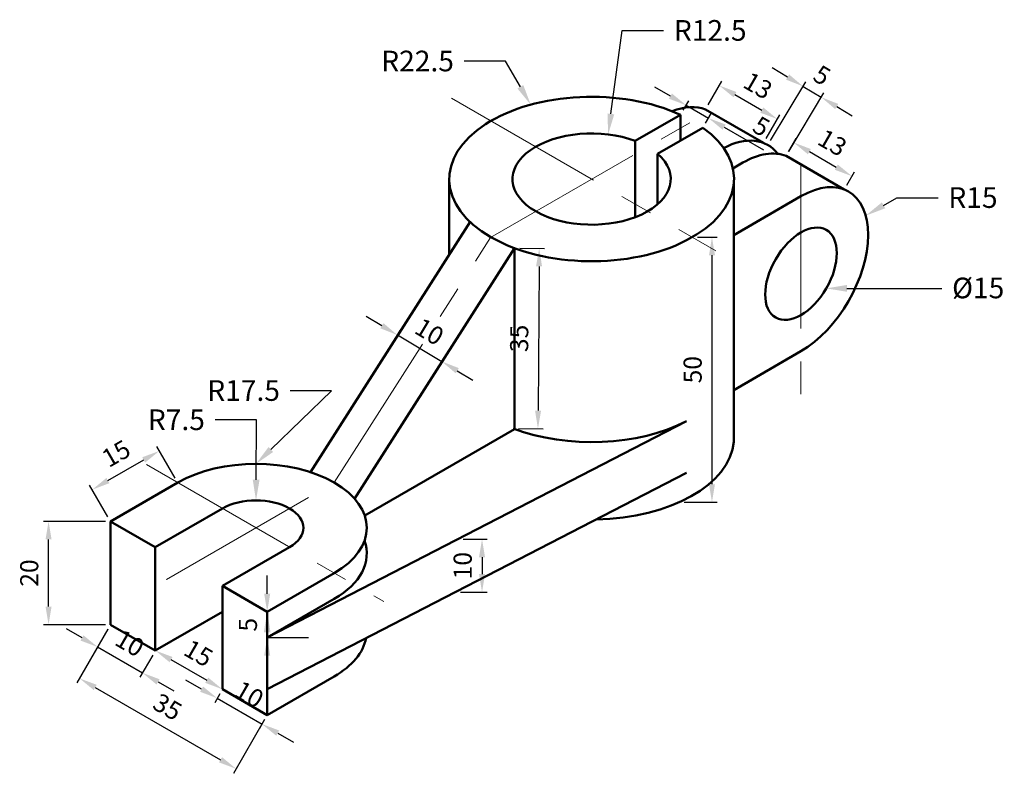
# Model space of a CAD drawing. Units: millimetres. Extents: x 2510 to 2700, y 1178 to 1324.
import ezdxf
from ezdxf import colors
from ezdxf.entities.mleader import LeaderData, LeaderLine
from ezdxf.math import Vec2, Vec3

# ---------------------------------------------------------------- set-up
doc = ezdxf.new("R2010")
doc.units = ezdxf.units.MM
doc.linetypes.add('CENTER', pattern=[50.8, 31.75, -6.35, 6.35, -6.35])
for name, color, linetype, lineweight in [('M-CNTR', 1, 'CENTER', 18), ('M-DIMS', 3, 'Continuous', 25), ('M-OUTL', 7, 'Continuous', 50)]:
    doc.layers.add(name, color=color, linetype=linetype, lineweight=lineweight)
doc.styles.get("Standard").update_dxf_attribs({"font": 'arial.ttf'})
doc.dimstyles.new('AM_ISO$0', dxfattribs={"dimtxt": 3.5, "dimasz": 3.5, "dimexe": 1, "dimexo": 1, "dimgap": 1.5, "dimtad": 1, "dimdsep": 46, "dimtxsty": 'Standard', "dimcen": 0, "dimclrd": 256, "dimclre": 256, "dimclrt": 2, "dimadec": 0, "dimazin": 2, "dimtp": 0.1, "dimtm": 0.1, "dimtfac": 0.71, "dimtdec": 3, "dimtmove": 0, "dimatfit": 3, "dimfxl": 1, "dimlwd": -1, "dimlwe": -1, "dimarcsym": 1})

# ---------------------------------------------------------------- blocks, each defined once
blk = doc.blocks.new('*D3')
at = {"layer": 'Defpoints', "color": 0, "transparency": 16777216}
for p in [(2640.08, 1281.6), (2637.52, 1230.3), (2643.88, 1230.3)]:
    blk.add_point(p, dxfattribs=at)
at = {"layer": 'M-DIMS', "color": 0, "linetype": 'ByBlock', "transparency": 16777216}
for p, q in [((2641.08, 1281.6), (2644.88, 1281.6)), ((2643.88, 1278.1), (2643.88, 1233.8)), ((2638.52, 1230.3), (2644.88, 1230.3))]:
    blk.add_line(p, q, dxfattribs=at)
at = {"layer": 'M-DIMS', "color": 0, "transparency": 16777216}
for points in [[(2643.3, 1278.1), (2644.46, 1278.1), (2643.88, 1281.6)], [(2643.3, 1233.8), (2644.46, 1233.8), (2643.88, 1230.3)]]:
    blk.add_solid(points, dxfattribs=at)
at = {"layer": 'M-DIMS', "color": 0, "transparency": 16777216, "insert": (2640.59, 1255.95), "char_height": 3.5, "attachment_point": 5, "rotation": 90}
blk.add_mtext('50', dxfattribs=at)
blk = doc.blocks.new('*D4')
at = {"layer": 'Defpoints', "color": 0, "transparency": 16777216}
for p in [(2605.68, 1279.48), (2605.44, 1244.57), (2610.2, 1244.53)]:
    blk.add_point(p, dxfattribs=at)
at = {"layer": 'M-DIMS', "color": 0, "linetype": 'ByBlock', "transparency": 16777216}
for p, q in [((2606.68, 1279.47), (2611.44, 1279.44)), ((2610.41, 1275.94), (2610.22, 1248.03)), ((2606.44, 1244.56), (2611.2, 1244.53))]:
    blk.add_line(p, q, dxfattribs=at)
at = {"layer": 'M-DIMS', "color": 0, "transparency": 16777216}
for points in [[(2609.83, 1275.95), (2611, 1275.94), (2610.44, 1279.44)], [(2609.64, 1248.04), (2610.81, 1248.03), (2610.2, 1244.53)]]:
    blk.add_solid(points, dxfattribs=at)
at = {"layer": 'M-DIMS', "color": 0, "transparency": 16777216, "insert": (2607.03, 1262.01), "char_height": 3.5, "attachment_point": 5, "rotation": 89.6095}
blk.add_mtext('35', dxfattribs=at)
blk = doc.blocks.new('*D5')
at = {"layer": 'Defpoints', "color": 0, "transparency": 16777216}
for p in [(2515.5, 1226.6), (2527.5, 1226.6), (2527.5, 1206.6)]:
    blk.add_point(p, dxfattribs=at)
at = {"layer": 'M-DIMS', "color": 0, "linetype": 'ByBlock', "transparency": 16777216}
for p, q in [((2526.5, 1226.6), (2514.5, 1226.6)), ((2515.5, 1210.1), (2515.5, 1223.1)), ((2526.5, 1206.6), (2514.5, 1206.6))]:
    blk.add_line(p, q, dxfattribs=at)
at = {"layer": 'M-DIMS', "color": 0, "transparency": 16777216}
for points in [[(2514.91, 1223.1), (2516.08, 1223.1), (2515.5, 1226.6)], [(2514.91, 1210.1), (2516.08, 1210.1), (2515.5, 1206.6)]]:
    blk.add_solid(points, dxfattribs=at)
at = {"layer": 'M-DIMS', "color": 0, "transparency": 16777216, "insert": (2512.21, 1216.6), "char_height": 3.5, "attachment_point": 5, "rotation": 90}
blk.add_mtext('20', dxfattribs=at)
blk = doc.blocks.new('*D6')
at = {"layer": 'Defpoints', "color": 0, "transparency": 16777216}
for p in [(2527.5, 1206.6), (2536.16, 1201.6), (2533.66, 1197.29)]:
    blk.add_point(p, dxfattribs=at)
at = {"layer": 'M-DIMS', "color": 0, "linetype": 'ByBlock', "transparency": 16777216}
for p, q in [((2521.97, 1204.04), (2518.94, 1205.79)), ((2527, 1205.74), (2524.5, 1201.42)), ((2525, 1202.29), (2533.66, 1197.29)), ((2535.66, 1200.74), (2533.16, 1196.42)), ((2536.69, 1195.54), (2539.73, 1193.79))]:
    blk.add_line(p, q, dxfattribs=at)
at = {"layer": 'M-DIMS', "color": 0, "transparency": 16777216}
for points in [[(2522.26, 1204.54), (2521.68, 1203.53), (2525, 1202.29)], [(2536.99, 1196.04), (2536.4, 1195.03), (2533.66, 1197.29)]]:
    blk.add_solid(points, dxfattribs=at)
at = {"layer": 'M-DIMS', "color": 0, "transparency": 16777216, "insert": (2530.98, 1202.63), "char_height": 3.5, "attachment_point": 5, "rotation": 330}
blk.add_mtext('10', dxfattribs=at)
blk = doc.blocks.new('*D7')
at = {"layer": 'Defpoints', "color": 0, "transparency": 16777216}
for p in [(2536.16, 1201.6), (2549.15, 1194.1), (2549.15, 1194.1)]:
    blk.add_point(p, dxfattribs=at)
at = {"layer": 'M-DIMS', "color": 0, "linetype": 'ByBlock', "transparency": 16777216}
blk.add_line((2539.19, 1199.85), (2546.12, 1195.85), dxfattribs=at)
at = {"layer": 'M-DIMS', "color": 0, "transparency": 16777216}
for points in [[(2539.48, 1200.36), (2538.9, 1199.35), (2536.16, 1201.6)], [(2546.41, 1196.36), (2545.82, 1195.35), (2549.15, 1194.1)]]:
    blk.add_solid(points, dxfattribs=at)
at = {"layer": 'M-DIMS', "color": 0, "transparency": 16777216, "insert": (2544.29, 1200.7), "char_height": 3.5, "attachment_point": 5, "rotation": 330}
blk.add_mtext('15', dxfattribs=at)
blk = doc.blocks.new('*D8')
at = {"layer": 'Defpoints', "color": 0, "transparency": 16777216}
for p in [(2549.15, 1194.1), (2557.81, 1189.1), (2556.81, 1187.37)]:
    blk.add_point(p, dxfattribs=at)
at = {"layer": 'M-DIMS', "color": 0, "linetype": 'ByBlock', "transparency": 16777216}
for p, q in [((2545.12, 1194.12), (2542.08, 1195.87)), ((2548.65, 1193.24), (2547.65, 1191.51)), ((2548.15, 1192.37), (2556.81, 1187.37)), ((2557.31, 1188.24), (2556.31, 1186.51)), ((2559.84, 1185.62), (2562.87, 1183.87))]:
    blk.add_line(p, q, dxfattribs=at)
at = {"layer": 'M-DIMS', "color": 0, "transparency": 16777216}
for points in [[(2545.41, 1194.63), (2544.82, 1193.62), (2548.15, 1192.37)], [(2560.13, 1186.13), (2559.55, 1185.12), (2556.81, 1187.37)]]:
    blk.add_solid(points, dxfattribs=at)
at = {"layer": 'M-DIMS', "color": 0, "transparency": 16777216, "insert": (2554.12, 1192.72), "char_height": 3.5, "attachment_point": 5, "rotation": 330}
blk.add_mtext('10', dxfattribs=at)
blk = doc.blocks.new('*D9')
at = {"layer": 'Defpoints', "color": 0, "transparency": 16777216}
for p in [(2527.5, 1206.6), (2557.81, 1189.1), (2551.81, 1178.71)]:
    blk.add_point(p, dxfattribs=at)
at = {"layer": 'M-DIMS', "color": 0, "linetype": 'ByBlock', "transparency": 16777216}
for p, q in [((2527, 1205.74), (2521, 1195.34)), ((2524.53, 1194.46), (2548.78, 1180.46)), ((2557.31, 1188.24), (2551.31, 1177.84))]:
    blk.add_line(p, q, dxfattribs=at)
at = {"layer": 'M-DIMS', "color": 0, "transparency": 16777216}
for points in [[(2524.82, 1194.97), (2524.24, 1193.96), (2521.5, 1196.21)], [(2549.07, 1180.97), (2548.48, 1179.96), (2551.81, 1178.71)]]:
    blk.add_solid(points, dxfattribs=at)
at = {"layer": 'M-DIMS', "color": 0, "transparency": 16777216, "insert": (2538.3, 1190.31), "char_height": 3.5, "attachment_point": 5, "rotation": 330}
blk.add_mtext('35', dxfattribs=at)
blk = doc.blocks.new('*D10')
at = {"layer": 'Defpoints', "color": 0, "transparency": 16777216}
for p in [(2536.94, 1240.24), (2540.49, 1234.1), (2527.5, 1226.6)]:
    blk.add_point(p, dxfattribs=at)
at = {"layer": 'M-DIMS', "color": 0, "linetype": 'ByBlock', "transparency": 16777216}
for p, q in [((2539.99, 1234.97), (2536.44, 1241.11)), ((2526.98, 1234.49), (2533.91, 1238.49)), ((2527, 1227.47), (2523.45, 1233.61))]:
    blk.add_line(p, q, dxfattribs=at)
at = {"layer": 'M-DIMS', "color": 0, "transparency": 16777216}
for points in [[(2533.62, 1239), (2534.2, 1237.99), (2536.94, 1240.24)], [(2526.69, 1235), (2527.27, 1233.99), (2523.95, 1232.74)]]:
    blk.add_solid(points, dxfattribs=at)
at = {"layer": 'M-DIMS', "color": 0, "transparency": 16777216, "insert": (2528.8, 1239.34), "char_height": 3.5, "attachment_point": 5, "rotation": 30}
blk.add_mtext('15', dxfattribs=at)
blk = doc.blocks.new('*D11')
at = {"layer": 'Defpoints', "color": 0, "transparency": 16777216}
for p in [(2581.62, 1260.35), (2591.59, 1257.55), (2590.2, 1255.23)]:
    blk.add_point(p, dxfattribs=at)
at = {"layer": 'M-DIMS', "color": 0, "linetype": 'ByBlock', "transparency": 16777216}
for p, q in [((2580, 1264.46), (2576.99, 1266.26)), ((2582.13, 1261.21), (2583.52, 1263.53)), ((2583, 1262.67), (2591.59, 1257.55)), ((2590.72, 1256.09), (2592.1, 1258.41)), ((2594.59, 1255.76), (2597.6, 1253.96))]:
    blk.add_line(p, q, dxfattribs=at)
at = {"layer": 'M-DIMS', "color": 0, "transparency": 16777216}
for points in [[(2580.3, 1264.96), (2579.7, 1263.96), (2583, 1262.67)], [(2594.89, 1256.26), (2594.29, 1255.26), (2591.59, 1257.55)]]:
    blk.add_solid(points, dxfattribs=at)
at = {"layer": 'M-DIMS', "color": 0, "transparency": 16777216, "insert": (2588.98, 1262.93), "char_height": 3.5, "attachment_point": 5, "rotation": 329.1839}
blk.add_mtext('10', dxfattribs=at)
blk = doc.blocks.new('*D12')
at = {"layer": 'Defpoints', "color": 0, "transparency": 16777216}
for p in [(2637.79, 1305.28), (2643.2, 1304.65), (2642.12, 1302.78)]:
    blk.add_point(p, dxfattribs=at)
at = {"layer": 'M-DIMS', "color": 0, "linetype": 'ByBlock', "transparency": 16777216}
for p, q in [((2635.84, 1308.9), (2632.81, 1310.65)), ((2638.29, 1306.15), (2639.37, 1308.01)), ((2638.87, 1307.15), (2643.2, 1304.65)), ((2642.62, 1303.65), (2643.7, 1305.51)), ((2646.23, 1302.9), (2653.87, 1298.49))]:
    blk.add_line(p, q, dxfattribs=at)
at = {"layer": 'M-DIMS', "color": 0, "transparency": 16777216}
for points in [[(2636.13, 1309.4), (2635.55, 1308.39), (2638.87, 1307.15)], [(2646.52, 1303.4), (2645.94, 1302.39), (2643.2, 1304.65)]]:
    blk.add_solid(points, dxfattribs=at)
at = {"layer": 'M-DIMS', "color": 0, "transparency": 16777216, "insert": (2653.21, 1302.66), "char_height": 3.5, "attachment_point": 5, "rotation": 330}
blk.add_mtext('5', dxfattribs=at)
blk = doc.blocks.new('*D13')
at = {"layer": 'Defpoints', "color": 0, "transparency": 16777216}
for p in [(2642.62, 1306.33), (2656.54, 1304.45), (2653.88, 1299.83)]:
    blk.add_point(p, dxfattribs=at)
at = {"layer": 'M-DIMS', "color": 0, "linetype": 'ByBlock', "transparency": 16777216}
for p, q in [((2643.12, 1307.19), (2645.79, 1311.81)), ((2648.32, 1309.2), (2653.51, 1306.2)), ((2654.38, 1300.69), (2657.04, 1305.31))]:
    blk.add_line(p, q, dxfattribs=at)
at = {"layer": 'M-DIMS', "color": 0, "transparency": 16777216}
for points in [[(2648.61, 1309.7), (2648.03, 1308.69), (2645.29, 1310.95)], [(2653.81, 1306.7), (2653.22, 1305.69), (2656.54, 1304.45)]]:
    blk.add_solid(points, dxfattribs=at)
at = {"layer": 'M-DIMS', "color": 0, "transparency": 16777216, "insert": (2652.56, 1310.54), "char_height": 3.5, "attachment_point": 5, "rotation": 330}
blk.add_mtext('13', dxfattribs=at)
blk = doc.blocks.new('*D14')
at = {"layer": 'Defpoints', "color": 0, "transparency": 16777216}
for p in [(2658.21, 1297.33), (2670.96, 1293.41), (2669.47, 1290.83)]:
    blk.add_point(p, dxfattribs=at)
at = {"layer": 'M-DIMS', "color": 0, "linetype": 'ByBlock', "transparency": 16777216}
for p, q in [((2658.71, 1298.19), (2660.2, 1300.77)), ((2662.73, 1298.16), (2667.92, 1295.16)), ((2669.97, 1291.69), (2671.46, 1294.27))]:
    blk.add_line(p, q, dxfattribs=at)
at = {"layer": 'M-DIMS', "color": 0, "transparency": 16777216}
for points in [[(2663.02, 1298.66), (2662.44, 1297.65), (2659.7, 1299.91)], [(2668.22, 1295.66), (2667.63, 1294.65), (2670.96, 1293.41)]]:
    blk.add_solid(points, dxfattribs=at)
at = {"layer": 'M-DIMS', "color": 0, "transparency": 16777216, "insert": (2666.97, 1299.5), "char_height": 3.5, "attachment_point": 5, "rotation": 330}
blk.add_mtext('13', dxfattribs=at)
blk = doc.blocks.new('*D15')
at = {"layer": 'Defpoints', "color": 0, "transparency": 16777216}
for p in [(2665.02, 1308.69), (2654.7, 1299.43), (2658.21, 1297.33)]:
    blk.add_point(p, dxfattribs=at)
at = {"layer": 'M-DIMS', "color": 0, "linetype": 'ByBlock', "transparency": 16777216}
for p, q in [((2658.51, 1312.59), (2655.51, 1314.39)), ((2655.21, 1300.29), (2662.03, 1311.65)), ((2658.72, 1298.19), (2665.54, 1309.55)), ((2661.51, 1310.79), (2665.02, 1308.69)), ((2668.02, 1306.89), (2671.02, 1305.09))]:
    blk.add_line(p, q, dxfattribs=at)
at = {"layer": 'M-DIMS', "color": 0, "transparency": 16777216}
for points in [[(2658.81, 1313.09), (2658.21, 1312.09), (2661.51, 1310.79)], [(2668.32, 1307.39), (2667.72, 1306.39), (2665.02, 1308.69)]]:
    blk.add_solid(points, dxfattribs=at)
at = {"layer": 'M-DIMS', "color": 0, "transparency": 16777216, "insert": (2664.95, 1312.55), "char_height": 3.5, "attachment_point": 5, "rotation": 329.0517}
blk.add_mtext('5', dxfattribs=at)
blk = doc.blocks.new('*D16')
at = {"layer": 'Defpoints', "color": 0, "transparency": 16777216}
for p in [(2557.81, 1209.1), (2557.81, 1204.1), (2557.81, 1204.1)]:
    blk.add_point(p, dxfattribs=at)
at = {"layer": 'M-DIMS', "color": 0, "linetype": 'ByBlock', "transparency": 16777216}
for p, q in [((2557.81, 1212.6), (2557.81, 1216.1)), ((2557.81, 1209.1), (2557.81, 1204.1)), ((2557.81, 1200.6), (2557.81, 1197.1))]:
    blk.add_line(p, q, dxfattribs=at)
at = {"layer": 'M-DIMS', "color": 0, "transparency": 16777216}
for points in [[(2557.22, 1212.6), (2558.39, 1212.6), (2557.81, 1209.1)], [(2557.22, 1200.6), (2558.39, 1200.6), (2557.81, 1204.1)]]:
    blk.add_solid(points, dxfattribs=at)
at = {"layer": 'M-DIMS', "color": 0, "transparency": 16777216, "insert": (2554.53, 1206.6), "char_height": 3.5, "attachment_point": 5, "rotation": 90}
blk.add_mtext('5', dxfattribs=at)
blk = doc.blocks.new('*D17')
at = {"layer": 'Defpoints', "color": 0, "transparency": 16777216}
for p in [(2594.74, 1223.17), (2594.22, 1212.9), (2599.38, 1212.9)]:
    blk.add_point(p, dxfattribs=at)
at = {"layer": 'M-DIMS', "color": 0, "linetype": 'ByBlock', "transparency": 16777216}
for p, q in [((2595.74, 1223.17), (2600.38, 1223.17)), ((2599.38, 1219.67), (2599.38, 1216.4)), ((2595.22, 1212.9), (2600.38, 1212.9))]:
    blk.add_line(p, q, dxfattribs=at)
at = {"layer": 'M-DIMS', "color": 0, "transparency": 16777216}
for points in [[(2598.8, 1219.67), (2599.96, 1219.67), (2599.38, 1223.17)], [(2598.8, 1216.4), (2599.96, 1216.4), (2599.38, 1212.9)]]:
    blk.add_solid(points, dxfattribs=at)
at = {"layer": 'M-DIMS', "color": 0, "transparency": 16777216, "insert": (2596.09, 1218.03), "char_height": 3.5, "attachment_point": 5, "rotation": 90}
blk.add_mtext('10', dxfattribs=at)

msp = doc.modelspace()

# ---------------------------------------------------------------- linework, layer by layer
at = {"layer": 'M-CNTR'}
for p, q in [((2593.463, 1308.517), (2644.631, 1278.975)), ((2601.048, 1281.569), (2644.807, 1306.764)), ((2661.103, 1274.522), (2661.103, 1295.657)), ((2661.103, 1295.657), (2661.103, 1247.756)), ((2570.769, 1234.119), (2601.048, 1281.569)), ((2534.454, 1237.586), (2580.376, 1211.073)), ((2538.321, 1215.353), (2570.769, 1234.119)), ((2555.641, 1225.353), (2538.321, 1215.353))]:
    msp.add_line(p, q, dxfattribs=at)
at = {"layer": 'M-OUTL'}
for p, q in [((2637.793, 1305.284), (2629.035, 1300.227)), ((2637.789, 1300.283), (2637.789, 1305.283)), ((2642.62, 1306.328), (2653.878, 1299.828)), ((2642.123, 1302.784), (2633.365, 1297.727)), ((2629.031, 1285.479), (2629.031, 1300.227)), ((2633.361, 1287.979), (2633.361, 1297.727)), ((2647.919, 1294.91), (2649.844, 1296.022)), ((2647.919, 1294.91), (2649.844, 1296.022)), ((2658.208, 1297.328), (2669.467, 1290.828)), ((2593.037, 1292.853), (2593.037, 1278.241)), ((2648.112, 1292.022), (2648.112, 1242.022)), ((2648.112, 1282.022), (2661.103, 1289.522)), ((2648.112, 1282.022), (2661.103, 1289.522)), ((2597.072, 1284.564), (2566.167, 1236.133)), ((2601.108, 1281.603), (2601.048, 1281.569)), ((2601.141, 1281.584), (2601.075, 1281.622)), ((2601.108, 1281.603), (2601.108, 1281.603)), ((2648.112, 1267.022), (2648.112, 1282.022)), ((2605.676, 1279.476), (2574.73, 1230.981)), ((2605.676, 1279.476), (2605.676, 1244.476)), ((2661.103, 1259.522), (2648.112, 1252.022)), ((2557.807, 1204.103), (2638.96, 1245.992)), ((2605.676, 1244.476), (2576.675, 1227.732)), ((2557.807, 1194.103), (2638.96, 1235.992)), ((2540.486, 1234.103), (2527.496, 1226.603)), ((2536.156, 1221.603), (2549.146, 1229.103)), ((2527.496, 1226.603), (2536.156, 1221.603)), ((2527.496, 1226.603), (2527.496, 1206.603)), ((2536.156, 1221.603), (2536.156, 1201.603)), ((2562.137, 1221.603), (2549.146, 1214.103)), ((2557.807, 1209.103), (2570.797, 1216.603)), ((2549.146, 1214.103), (2557.807, 1209.103)), ((2549.146, 1214.103), (2549.146, 1194.103)), ((2557.807, 1204.103), (2570.797, 1211.603)), ((2536.156, 1201.603), (2549.146, 1209.103)), ((2557.807, 1209.103), (2557.807, 1189.103)), ((2557.807, 1209.103), (2557.807, 1204.103)), ((2527.496, 1206.603), (2536.156, 1201.603)), ((2557.807, 1189.103), (2570.797, 1196.603)), ((2549.146, 1194.103), (2557.807, 1189.103)), ((2557.807, 1189.103), (2557.807, 1194.103))]:
    msp.add_line(p, q, dxfattribs=at)
for centre, major_axis, start_param, end_param in [((2620.593, 1292.853), (-27.557, 0), 4.0383318, 10.0988351), ((2634.256, 1290.022), (-9.186, -15.91), 3.2274705, 3.7777064), ((2620.593, 1292.853), (-15.309, 0), 4.1283487, 10.0088182), ((2645.514, 1283.522), (-9.186, -15.91), 2.9036515, 3.880685), ((2649.844, 1281.022), (-9.186, -15.91), 3.2274705, 3.9269908), ((2661.103, 1274.522), (-9.186, -15.91), 0.7853982, 3.9269908), ((2620.593, 1257.853), (-27.557, 0), 7.2716504, 8.5834916), ((2620.593, 1242.853), (-15.309, 0), 9.5899664, 9.6144754), ((2620.593, 1242.853), (-27.557, 0), 7.8848422, 9.3724911), ((2555.641, 1225.353), (-21.433, 0), 2.3561945, 5.4977871), ((2555.641, 1225.353), (-9.186, 0), 2.3561945, 5.4977871), ((2555.641, 1220.353), (-21.433, 0), 2.3561945, 3.3450234), ((2555.638, 1205.353), (21.433, 0), 5.4977871, 6.1720255)]:
    msp.add_ellipse(centre, major_axis=major_axis, ratio=0.5773503, start_param=start_param, end_param=end_param, dxfattribs=at)
msp.add_ellipse((2661.103, 1274.522), major_axis=(-4.899, -8.485), ratio=0.5773503, dxfattribs=at)

# ---------------------------------------------------------------- dimensions: what is measured, and where the dimension line sits
at = {"layer": 'M-DIMS'}
for base, p1, p2, angle, text, override, picture, middle in [((2665.021, 1308.69), (2654.7, 1299.432), (2658.208, 1297.328), 329.05172, '5', {"dimclrd": 0, "dimclre": 0, "dimclrt": 0}, '*D15', (2663.267, 1309.742)), ((2591.587, 1257.55), (2581.619, 1260.349), (2590.203, 1255.229), 329.1839, '10', {"dimpost": '', "dimclrd": 0, "dimclre": 0, "dimclrt": 0}, '*D11', (2587.296, 1260.11))]:
    dim = msp.add_linear_dim(base=base, p1=p1, p2=p2, angle=angle, text=text, dimstyle='AM_ISO$0', override=override, dxfattribs=at)
    dim.commit()
    dim.dimension.update_dxf_attribs({"geometry": picture, "text_midpoint": middle, "dimtype": 161})
for p1, p2, distance, override, picture, middle in [((2642.62, 1306.328), (2653.878, 1299.828), 5.333, {"dimclrd": 0, "dimclre": 0, "dimclrt": 0}, '*D13', (2652.56, 1310.544)), ((2637.793, 1305.284), (2642.123, 1302.784), 2.152, {"dimpost": '', "dimclrd": 0, "dimclre": 0, "dimclrt": 0}, '*D12', (2653.205, 1302.658)), ((2658.208, 1297.328), (2669.467, 1290.828), 2.977, {"dimclrd": 0, "dimclre": 0, "dimclrt": 0}, '*D14', (2666.97, 1299.504)), ((2527.496, 1226.603), (2540.486, 1234.103), 7.091, {"dimclrd": 0, "dimclre": 0, "dimclrt": 0}, '*D10', (2528.802, 1239.341)), ((2527.496, 1206.603), (2527.496, 1226.603), 12, {"dimclrd": 0, "dimclre": 0, "dimclrt": 0}, '*D5', (2512.209, 1216.603)), ((2527.496, 1206.603), (2536.156, 1201.603), -4.984, {"dimclrd": 0, "dimclre": 0, "dimclrt": 0}, '*D6', (2530.977, 1202.633)), ((2527.496, 1206.603), (2557.807, 1189.103), -12, {"dimpost": '', "dimclrd": 0, "dimclre": 0, "dimclrt": 0}, '*D9', (2538.295, 1190.309)), ((2536.156, 1201.603), (2549.146, 1194.103), 0, {"dimpost": '', "dimclrd": 0, "dimclre": 0, "dimclrt": 0}, '*D7', (2544.295, 1200.7)), ((2549.146, 1194.103), (2557.807, 1189.103), -2, {"dimclrd": 0, "dimclre": 0, "dimclrt": 0}, '*D8', (2554.12, 1192.718))]:
    dim = msp.add_aligned_dim(p1=p1, p2=p2, distance=distance, dimstyle='AM_ISO$0', override=override, dxfattribs=at)
    dim.commit()
    dim.dimension.update_dxf_attribs({"geometry": picture, "text_midpoint": middle})
for base, p1, p2, text, picture, middle in [((2643.879, 1230.301), (2640.079, 1281.603), (2637.525, 1230.301), '50', '*D3', (2640.592, 1255.952)), ((2599.381, 1212.898), (2594.737, 1223.166), (2594.218, 1212.898), '10', '*D17', (2596.094, 1218.032))]:
    dim = msp.add_linear_dim(base=base, p1=p1, p2=p2, angle=90, text=text, dimstyle='AM_ISO$0', override={"dimpost": '', "dimclrd": 0, "dimclre": 0, "dimclrt": 0}, dxfattribs=at)
    dim.commit()
    dim.dimension.update_dxf_attribs({"geometry": picture, "text_midpoint": middle})
dim = msp.add_aligned_dim(p1=(2605.676, 1279.476), p2=(2605.438, 1244.566), distance=4.76, text='35', dimstyle='AM_ISO$0', override={"dimpost": '', "dimclrd": 0, "dimclre": 0, "dimclrt": 0}, dxfattribs=at)
dim.commit()
dim.dimension.update_dxf_attribs({"geometry": '*D4', "text_midpoint": (2607.029, 1262.011)})
dim = msp.add_linear_dim(base=(2557.807, 1204.103), p1=(2557.807, 1209.103), p2=(2557.807, 1204.103), angle=90, dimstyle='AM_ISO$0', override={"dimclrd": 0, "dimclre": 0, "dimclrt": 0}, dxfattribs=at)
dim.commit()
dim.dimension.update_dxf_attribs({"geometry": '*D16', "text_midpoint": (2557.807, 1206.603), "dimtype": 160})

# ---------------------------------------------------------------- leaders
ml = msp.add_multileader_mtext('Standard', dxfattribs=at)
ml.set_content('{\\C2;R12.5}', color=256)
ml.set_leader_properties()
ml.build(insert=Vec2(0, 0))
ctx = ml.context
ctx.base_point, ctx.plane_origin = Vec3(2634.507, 1321.585), Vec3(2623.78, 1301.498)
notes = []
notes.append((ctx, [(0, (1, 1, 0), (2626.507, 1321.585), (1, 0), 8, [(0, [(2623.78, 1301.498)], 0, [])])]))
ctx.mtext.insert, ctx.mtext.flow_direction = Vec3(2636.507, 1323.619), 5
ml = msp.add_multileader_mtext('Standard', dxfattribs=at)
ml.set_content('{\\C2;R22.5}', color=256)
ml.set_leader_properties()
ml.build(insert=Vec2(0, 0))
ctx = ml.context
ctx.base_point, ctx.plane_origin = Vec3(2577.695, 1315.659), Vec3(2608.807, 1307.234)
ctx.text_align_type = 2
notes.append((ctx, [(0, (1, 1, 0), (2603.943, 1315.659), (-1, 0), 8, [(0, [(2608.807, 1307.234)], 0, [])])]))
ctx.mtext.insert, ctx.mtext.alignment, ctx.mtext.flow_direction = Vec3(2593.943, 1317.693), 3, 5
ml = msp.add_multileader_mtext('Standard', dxfattribs=at)
ml.set_content('{\\C2;R15}', color=256)
ml.set_leader_properties()
ml.build(insert=Vec2(0, 0))
ctx = ml.context
ctx.base_point, ctx.plane_origin = Vec3(2687.627, 1289.232), Vec3(2673.619, 1285.763)
notes.append((ctx, [(0, (1, 1, 0), (2679.627, 1289.232), (1, 0), 8, [(0, [(2673.619, 1285.763)], 0, [])])]))
ctx.mtext.insert, ctx.mtext.flow_direction = Vec3(2689.627, 1291.266), 5
ml = msp.add_multileader_mtext('Standard', dxfattribs=at)
ml.set_content('{\\C2;%%C15}', color=256)
ml.set_leader_properties()
ml.build(insert=Vec2(0, 0))
ctx = ml.context
ctx.base_point, ctx.plane_origin = Vec3(2688.342, 1271.693), Vec3(2666.002, 1271.693)
notes.append((ctx, [(0, (1, 1, 0), (2680.342, 1271.693), (1, 0), 8, [(0, [(2666.002, 1271.693)], 0, [])])]))
ctx.mtext.insert, ctx.mtext.flow_direction = Vec3(2690.342, 1273.774), 5
ml = msp.add_multileader_mtext('Standard', dxfattribs=at)
ml.set_content('{\\C2;R17.5}', color=256)
ml.set_leader_properties()
ml.build(insert=Vec2(0, 0))
ctx = ml.context
ctx.base_point, ctx.plane_origin = Vec3(2544.028, 1251.891), Vec3(2555.641, 1237.728)
ctx.text_align_type = 2
notes.append((ctx, [(0, (1, 1, 0), (2570.277, 1251.891), (-1, 0), 8, [(0, [(2555.641, 1237.728)], 0, [])])]))
ctx.mtext.insert, ctx.mtext.alignment, ctx.mtext.flow_direction = Vec3(2560.277, 1253.925), 3, 5
ml = msp.add_multileader_mtext('Standard', dxfattribs=at)
ml.set_content('{\\C2;R7.5}', color=256)
ml.set_leader_properties()
ml.build(insert=Vec2(0, 0))
ctx = ml.context
ctx.base_point, ctx.plane_origin = Vec3(2532.611, 1246.24), Vec3(2555.641, 1230.657)
ctx.text_align_type = 2
notes.append((ctx, [(0, (1, 1, 0), (2555.752, 1246.24), (-1, 0), 8, [(0, [(2555.641, 1230.657)], 0, [])])]))
ctx.mtext.insert, ctx.mtext.alignment, ctx.mtext.flow_direction = Vec3(2545.752, 1248.275), 3, 5
ml = msp.add_multileader_mtext('Standard', dxfattribs=at)
ml.set_content('', color=256)
ml.set_leader_properties()
ml.build(insert=Vec2(0, 0))
ctx = ml.context
ctx.base_point, ctx.plane_origin = Vec3(2565.807, 1204.103), Vec3(2557.807, 1209.103)
notes.append((ctx, [(0, (1, 1, 0), (2557.807, 1204.103), (1, 0), 8, [(0, [(2557.807, 1209.103)], 0, [])])]))
ctx.mtext.insert, ctx.mtext.flow_direction = Vec3(2567.807, 1206.103), 5
for ctx, leaders in notes:
    for number, flags, end, landing, length, lines in leaders:
        leader = LeaderData()
        leader.index, (leader.has_last_leader_line, leader.has_dogleg_vector, leader.attachment_direction) = number, flags
        leader.last_leader_point, leader.dogleg_vector, leader.dogleg_length = Vec3(end), Vec3(landing), length
        for number, points, colour, breaks in lines:
            line = LeaderLine()
            line.index, line.vertices, line.color, line.breaks = number, Vec3.list(points), colors.encode_raw_color(colour), breaks
            leader.lines.append(line)
        ctx.leaders.append(leader)

doc.saveas('drawing.dxf')
